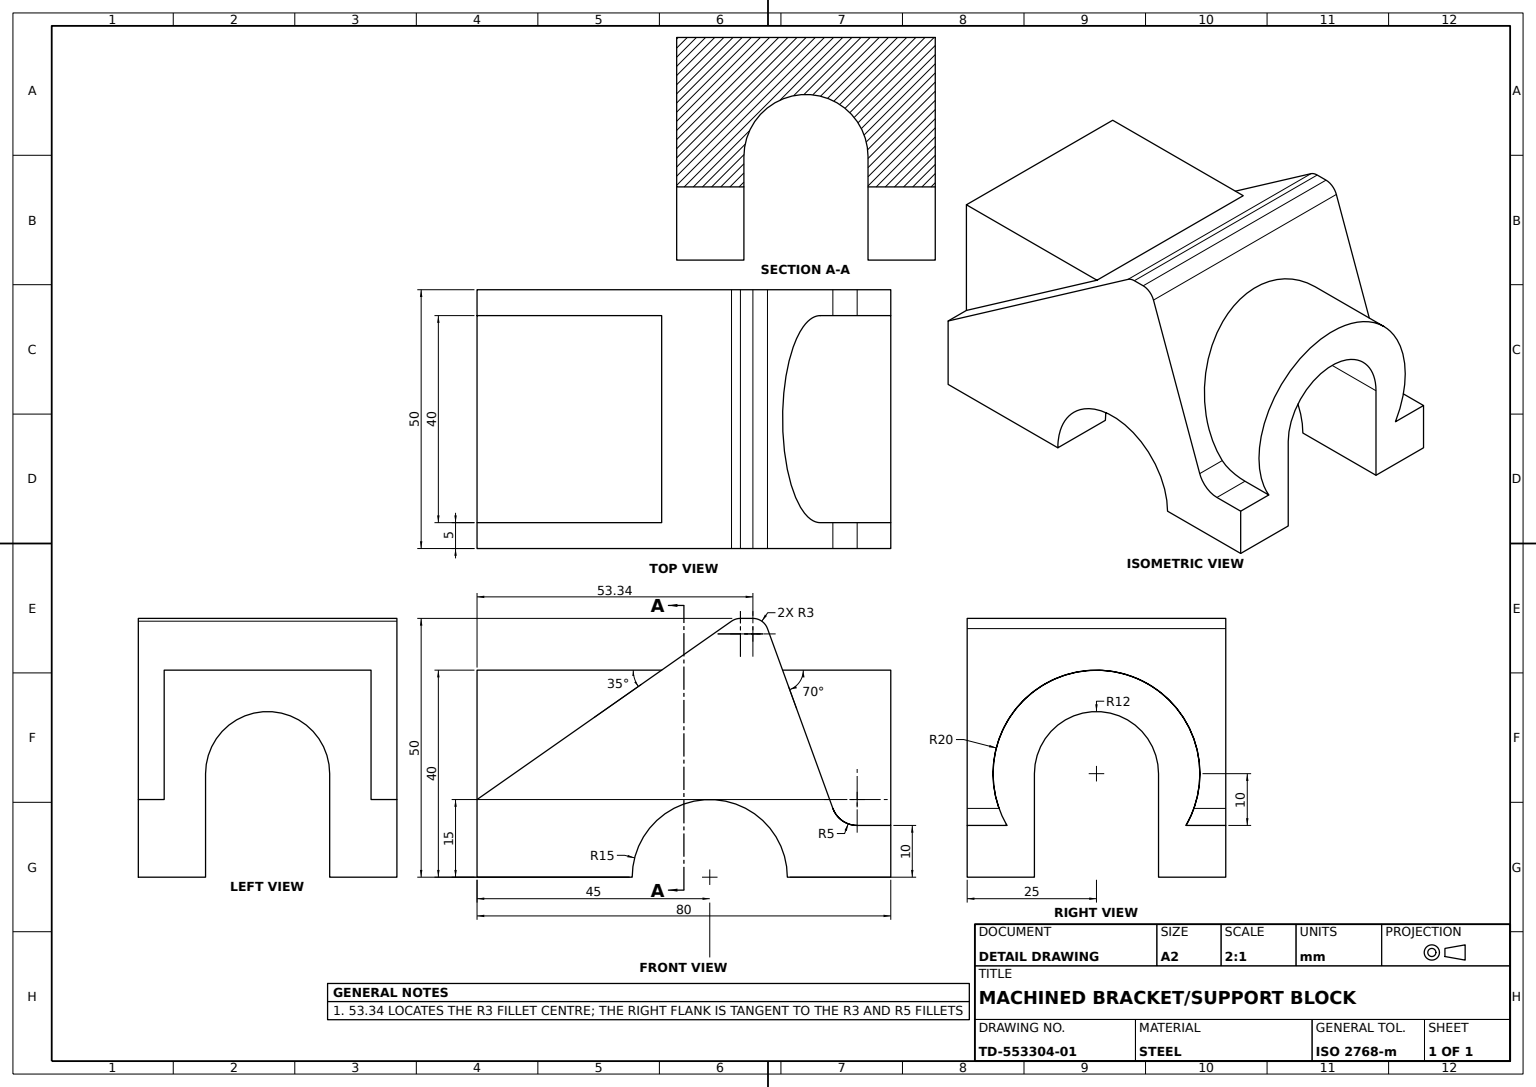
from build123d import *

# Parameters (mm, degrees)
BASE_BLOCK_DEPTH         = 25
TOWER_SKETCH_40X40_W     = 40
TOWER_SKETCH_40X40_H     = 40
TOWER_BLOCK_DEPTH        = 55
RIDGE_SADDLE_BODY_DEPTH  = 25
RIDGE_FILLET_R3_R        = 3
SADDLE_OPENING_CUT_DEPTH = 90.022469074
RIDGE_GROOVE_CUT_DEPTH   = 99.994949366
EDGE_FILLET_R5_R         = 5


with BuildPart() as part:
    # Base Profile Sketch → Base Block (new body)
    with BuildSketch(Plane(origin=(0, 0, 0), x_dir=(0, 0, -1), z_dir=(1, 0, 0))):
        with BuildLine():
            Line((-17.320508076, -10), (-25, -10))
            Line((-25, -10), (-25, -20))
            Line((-25, -20), (-12, -20))
            Line((-12, -20), (-12, 0))
            ThreePointArc((-12, 0), (0, 12), (12, 0))
            Line((12, 0), (12, -20))
            Line((12, -20), (25, -20))
            Line((25, -20), (25, -10))
            Line((25, -10), (17.320508076, -10))
            ThreePointArc((17.320508076, -10), (0, 20), (-17.320508076, -10))
        make_face()
    extrude(amount=-BASE_BLOCK_DEPTH)

    # Tower Sketch 40x40 → Tower Block (add)
    with BuildSketch(Plane.ZY.offset(25)):
        Rectangle(TOWER_SKETCH_40X40_W, TOWER_SKETCH_40X40_H)
    extrude(amount=TOWER_BLOCK_DEPTH)

    # Ridge Profile Sketch → Ridge Saddle Body (add, symmetric)
    with BuildSketch(Plane.XY):
        Polygon((-80, -4.997409114), (-30.018519933, 30), (-24.56, 30), (-10.001190629, -10), (0, -10), (0, -20), (-80, -20), align=None)
    extrude(amount=RIDGE_SADDLE_BODY_DEPTH, both=True)

    # Ridge Fillet R3
    ridge_fillet_r3_edges = [part.edges().sort_by_distance(p)[0] for p in [
        (-30.018519933, 30, 0),
        (-24.56, 30, 0),
    ]]
    fillet(ridge_fillet_r3_edges, radius=RIDGE_FILLET_R3_R)

    # Saddle Opening Sketch → Saddle Opening Cut (cut, through all)
    with BuildSketch(Plane(origin=(0, 0, 0), x_dir=(0, 0, -1), z_dir=(1, 0, 0))):
        with BuildLine():
            Line((12, 0), (12, -10))
            Line((12, -10), (12, -20))
            Line((12, -20), (-12, -20))
            Line((-12, -20), (-12, -10))
            Line((-12, -10), (-12, 0))
            ThreePointArc((-12, 0), (0, 12), (12, 0))
        make_face()
    extrude(amount=-SADDLE_OPENING_CUT_DEPTH, mode=Mode.SUBTRACT)

    # Ridge Groove Sketch → Ridge Groove Cut (cut, through all)
    with BuildSketch(Plane.XY.offset(25)):
        with BuildLine():
            Line((-50, -20), (-20, -20))
            ThreePointArc((-20, -20), (-35, -5), (-50, -20))
        make_face()
    extrude(amount=-RIDGE_GROOVE_CUT_DEPTH, mode=Mode.SUBTRACT)

    # Edge Fillet R5
    edge_fillet_r5_edges = [part.edges().sort_by_distance(p)[0] for p in [
        (-10.001190629, -10, -21.160254038),
        (-10.001190629, -10, 21.160254038),
    ]]
    fillet(edge_fillet_r5_edges, radius=EDGE_FILLET_R5_R)


solid = part.part
